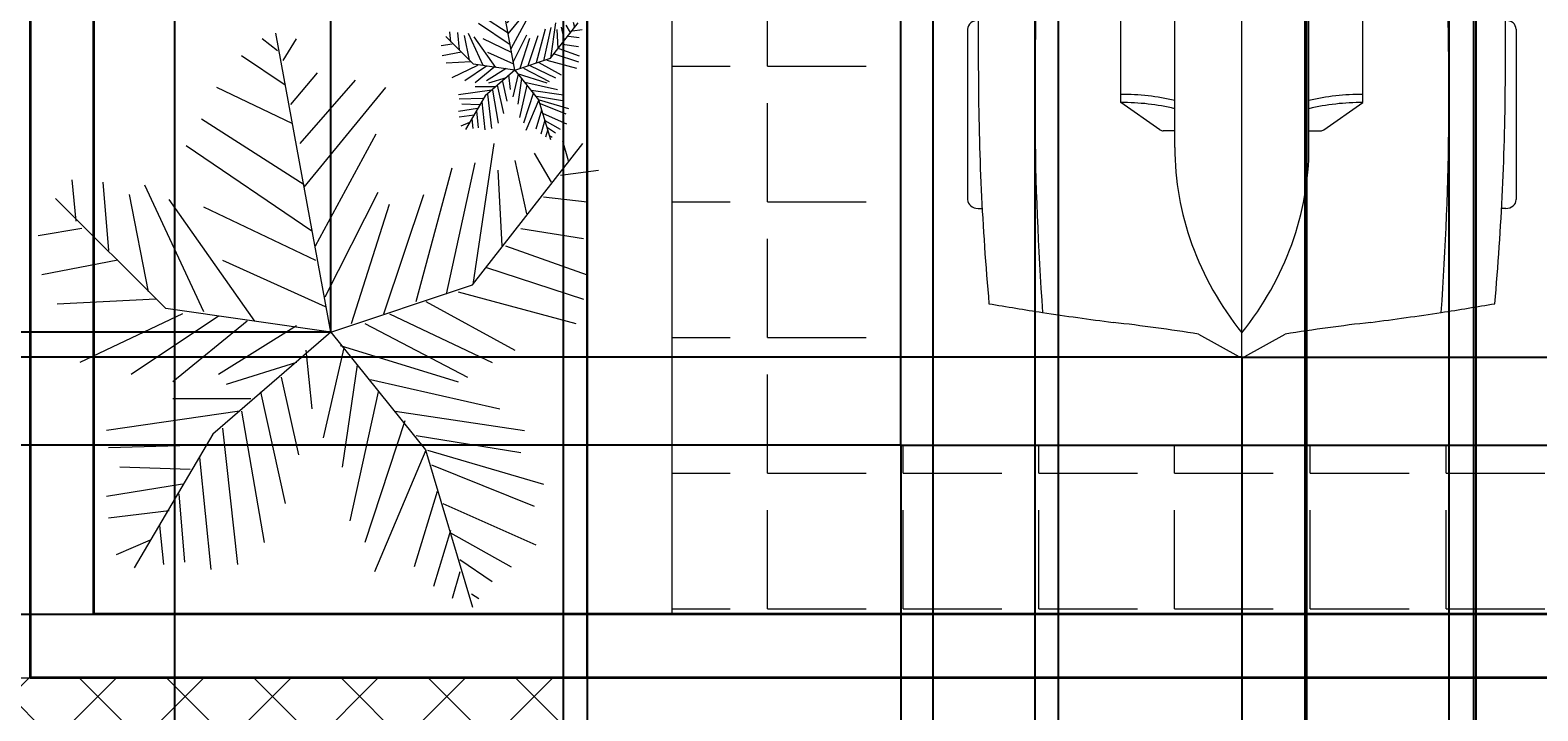
# Model space of a CAD drawing. Units: inches. Extents: x 818 to 1898, y 976 to 2364.
# Tile 3 of 96: x 993 to 1207, y 1198 to 1295. Entities that reach past the tile are written whole.
import ezdxf

# ---------------------------------------------------------------- set-up
doc = ezdxf.new("R2010")
doc.units = ezdxf.units.IN
doc.header["$LTSCALE"] = 5
doc.header["$MEASUREMENT"] = 0
for name, color, linetype, lineweight in [('A-ANNO-DIMS', 2, 'Continuous', 18), ('C-PAVE-PATT', 8, 'Continuous', 9), ('C-PKNG', 8, 'Continuous', 18), ('C-PKNG-PATT', 9, 'Continuous', 9), ('C-PROP', 7, 'Continuous', 35), ('L-PAVE', 8, 'Continuous', 18), ('L-PLNT-BEDS', 94, 'Continuous', 18)]:
    doc.layers.add(name, color=color, linetype=linetype, lineweight=lineweight)
doc.layers.add('L-PLNT', color=116, linetype='Continuous', lineweight=13, true_color=0x136734)
doc.styles.get("Standard").update_dxf_attribs({"font": 'arial.ttf'})
doc.dimstyles.get("Standard").update_dxf_attribs({"dimtxt": 0.18, "dimasz": 0.18, "dimexe": 0.18, "dimexo": 0.0625, "dimgap": 0.09, "dimtad": 0, "dimtih": 1, "dimtoh": 1, "dimdec": 4, "dimzin": 0, "dimdsep": 46, "dimtxsty": 'Standard', "dimcen": 0.09, "dimadec": 0, "dimazin": 0, "dimtfac": 1, "dimtdec": 4, "dimtofl": 0, "dimtmove": 0, "dimatfit": 3, "dimfxl": 1, "dimtolj": 1, "dimtzin": 0, "dimarcsym": 0})
pattern_1 = [(0, (0, 0), (0, 19.25), [14, -5.25]), (90, (0, 0), (-19.25, 1e-15), [14, -5.25])]

# ---------------------------------------------------------------- blocks, each defined once
blk = doc.blocks.new('*U13')
for p, q in [((46.55, 38.89), (22.35, 38.89)), ((136.7, 38.89), (160.9, 38.89)), ((21.1, 37.41), (21.1, 36.83)), ((47.8, 37.39), (47.8, 37.41)), ((135.45, 37.07), (135.45, 37.41)), ((162.15, 37.41), (162.15, 36.77)), ((87.99, 31.87), (74.76, 35.92)), ((134.31, 35.6), (119.29, 31.78)), ((186.47, -33.5), (186.47, 33.5)), ((188.4, -32.76), (188.4, 32.76)), ((70.03, 31.54), (86.41, 29.35)), ((138.42, 29.35), (157.25, 29.35)), ((186.47, 29.35), (167.01, 29.35)), ((164.52, 26.39), (164.52, -26.39)), ((32.27, 11.63), (36.13, 17.17)), ((36.13, 17.17), (50.94, 17.17)), ((32.12, 9.51), (32.12, 11.15)), ((58.92, -10.77), (58.92, 10.77)), ((29.77, 9.51), (51.68, 9.51)), ((66.55, -10.53), (66.55, 10.53)), ((186.47, -10.53), (186.47, 10.53)), ((82.74, 8.5), (82.74, -8.5)), ((3.27, 6.13), (0.1, 0.41)), ((0, 0), (51.68, 0)), ((0.1, -0.41), (3.27, -6.13)), ((29.77, -9.51), (51.68, -9.51)), ((32.12, -9.51), (32.12, -11.15)), ((32.27, -11.63), (36.13, -17.17)), ((36.13, -17.17), (50.94, -17.17)), ((86.41, -29.35), (70.03, -31.54)), ((157.25, -29.35), (138.42, -29.35)), ((167.01, -29.35), (186.47, -29.35)), ((87.99, -31.87), (74.76, -35.92)), ((134.31, -35.6), (119.29, -31.78)), ((21.1, -37.41), (21.1, -36.83)), ((47.8, -37.39), (47.8, -37.41)), ((135.45, -37.07), (135.45, -37.41)), ((162.15, -37.41), (162.15, -36.77)), ((46.55, -38.89), (22.35, -38.89)), ((136.7, -38.89), (160.9, -38.89))]:
    blk.add_line(p, q)
for centre, major_axis, ratio, start_param, end_param in [((22.35, 37.41), (0, -1.48), 0.842304, 3.141593, 4.712389), ((46.55, 37.41), (0, 1.48), 0.842304, -1.570796, 0), ((136.7, 37.41), (0, -1.48), 0.842304, 3.141593, 4.712389), ((160.9, 37.41), (0, 1.48), 0.842304, -1.570796, 0), ((41.19, -490.86), (0, 528.23), 0.842304, 0.00281, 0.075598), ((64.48, -10555.62), (0, 10593.03), 0.842304, -0.013397, 0.002797), ((180.63, 35.84), (0, 2.22), 0.842304, -0.013017, 1.249894), ((64.48, -10556.36), (0, 10595.31), 0.842304, -0.013397, -0.013017), ((183.98, 33.5), (0, -2.96), 0.842304, 1.570796, 3.128196), ((183.98, 32.76), (0, -5.25), 0.842304, 1.570796, 3.128196), ((266.03, -27.52), (0, 313.31), 0.842304, 1.367076, 1.39176), ((64.48, -10555.62), (0, -10591.55), 0.842304, 3.133765, 3.140441), ((135.29, 5.39), (0, 81.77), 0.842304, 1.245306, 1.50788), ((95.79, -3666.35), (0, -3698.24), 0.842304, 3.134049, 3.144098), ((259.18, -27.52), (0, -305.3), 0.842304, 4.528606, 4.561838), ((37.47, -593.96), (0, -623.33), 0.842304, 3.096046, 3.200911), ((134.4, 5.39), (0, -89.78), 0.842304, 4.449482, 4.652344), ((149.6, 2.8), (0, -79.58), 0.842304, 4.372215, 4.640744), ((17.08, 0), (0, 147.02), 0.842304, 4.511394, 4.913384), ((35.91, 0), (0, 147.02), 0.842304, 4.511394, 4.913384), ((167.01, 26.39), (0, 2.96), 0.842304, 0, 1.570796), ((-204.49, 52.4), (0, -250.96), 0.842304, 1.385369, 1.434372), ((13.04, 17.01), (0, 27.42), 0.842304, 4.435146, 4.718221), ((14.2, 17.01), (0, 27.42), 0.842304, 4.435146, 4.718221), ((50.79, 13.34), (6.34, -0.36), 0.603834, -1.395552, 1.581315), ((32.75, 11.15), (0, 0.74), 0.842304, 0.879714, 1.570796), ((29.77, -46.66), (0, 56.17), 0.842304, 0, 0.590319), ((0.62, 0), (0, -0.74), 0.842304, 4.131459, 5.293319), ((29.77, 46.66), (0, 56.17), 0.842304, 2.551274, 3.141593), ((-204.49, -52.4), (0, 250.96), 0.842304, -1.434372, -1.385369), ((149.6, -2.8), (0, -79.58), 0.842304, -1.499151, -1.230623), ((13.04, -17.01), (0, -27.42), 0.842304, 1.564964, 1.848039), ((14.2, -17.01), (0, -27.42), 0.842304, 1.564964, 1.848039), ((135.29, -5.39), (0, -81.77), 0.842304, -1.50788, -1.245306), ((32.75, -11.15), (0, -0.74), 0.842304, 4.712389, 5.403472), ((134.4, -5.39), (0, -89.78), 0.842304, -1.510751, -1.307889), ((259.18, 27.52), (0, 305.3), 0.842304, 1.721348, 1.754579), ((167.01, -26.39), (0, -2.96), 0.842304, 4.712389, 6.283185), ((266.03, 27.52), (0, 313.31), 0.842304, 1.749832, 1.774517), ((37.47, 593.96), (0, -623.33), 0.842304, -0.059319, 0.045547), ((95.79, 3666.35), (0, -3698.24), 0.842304, -0.002505, 0.007544), ((183.98, -33.5), (0, 2.96), 0.842304, 3.15499, 4.712389), ((183.98, -32.76), (0, -5.25), 0.842304, 0.013397, 1.570796), ((41.19, 490.86), (0, -528.23), 0.842304, -0.075598, -0.00281), ((64.48, 10555.62), (0, -10591.55), 0.842304, 0.001152, 0.007828), ((22.35, -37.41), (0, 1.48), 0.842304, 1.570796, 3.141593), ((64.48, 10555.62), (0, 10593.03), 0.842304, 3.138796, 3.15499), ((46.55, -37.41), (0, -1.48), 0.842304, 0, 1.570796), ((136.7, -37.41), (0, -1.48), 0.842304, -1.570796, 0), ((160.9, -37.41), (0, 1.48), 0.842304, 3.141593, 4.712389), ((180.63, -35.84), (0, -2.22), 0.842304, -1.249894, 0.013017), ((64.48, 10556.36), (0, 10595.31), 0.842304, 3.15461, 3.15499)]:
    blk.add_ellipse(centre, major_axis=major_axis, ratio=ratio, start_param=start_param, end_param=end_param)
at = {"extrusion": (0, 0, -1)}
blk.add_ellipse((50.79, -13.34), major_axis=(6.34, 0.36), ratio=0.603834, start_param=-1.395552, end_param=1.581315, dxfattribs=at)
blk = doc.blocks.new('SHRUB-ACCENT')
for p, q in [((8.8, 18.63), (7.25, 19.67)), ((8.53, 19.84), (7.99, 20.28)), ((10.44, 9.82), (8.47, 20.47)), ((8.74, 19.5), (9.21, 20.28)), ((9.48, 15.07), (5.82, 17.41)), ((9.08, 17.24), (6.37, 18.54)), ((9.01, 17.93), (9.96, 19.06)), ((9.35, 16.54), (11.31, 18.8)), ((9.48, 14.98), (12.39, 18.54)), ((1.35, 13.77), (1.22, 15.24)), ((2.3, 15.16), (2.51, 12.72)), ((3.79, 15.07), (5.89, 10.55)), ((9.75, 13.42), (5.28, 16.46)), ((9.89, 12.9), (12.06, 16.89)), ((13.48, 10.9), (14.76, 15.68)), ((14.56, 11.16), (15.58, 15.85)), ((15.49, 11.5), (19.41, 16.55)), ((15.51, 11.51), (16.25, 16.54)), ((16.39, 15.59), (16.53, 12.9)), ((17, 15.94), (17.41, 14.03)), ((17.68, 16.2), (18.29, 15.16)), ((18.62, 15.42), (19.98, 15.59)), ((18.69, 16.63), (18.9, 15.94)), ((1.56, 13.51), (0, 13.25)), ((4.55, 10.66), (0.62, 14.58)), ((3.25, 14.72), (3.93, 11.25)), ((7.72, 10.21), (4.67, 14.55)), ((5.89, 14.29), (9.89, 12.38)), ((10.23, 11.07), (12.12, 14.81)), ((11.17, 10.12), (12.53, 14.37)), ((12.33, 10.47), (13.75, 14.72)), ((16.66, 12.9), (19.57, 11.86)), ((17.2, 13.51), (19.44, 13.16)), ((18.02, 14.63), (19.57, 14.46)), ((2.84, 12.38), (0.14, 11.86)), ((4.2, 10.99), (0.68, 10.81)), ((6.57, 12.38), (10.23, 10.73)), ((10.44, 9.82), (15.49, 11.5)), ((13.82, 10.9), (17, 9.16)), ((14.97, 11.25), (19.17, 10.12)), ((15.98, 12.12), (19.44, 10.99)), ((5.15, 10.47), (1.49, 8.73)), ((6.43, 10.38), (3.32, 8.3)), ((10.44, 9.82), (4.55, 10.66)), ((7.45, 10.21), (4.81, 8.04)), ((10.44, 9.82), (6.23, 6.17)), ((9.21, 10.03), (6.43, 8.3)), ((9.21, 8.73), (6.7, 7.95)), ((9.55, 9.16), (9.75, 7.08)), ((10.9, 9.25), (10.16, 6.04)), ((10.44, 9.82), (13.8, 5.61)), ((10.77, 9.34), (14.97, 8.04)), ((11.38, 8.64), (10.84, 5)), ((11.65, 10.12), (15.31, 8.21)), ((12.53, 10.47), (16.19, 8.73)), ((7.18, 6.99), (2.44, 6.3)), ((7.59, 7.43), (4.81, 7.43)), ((7.25, 6.99), (8.06, 2.31)), ((7.92, 7.69), (8.8, 3.69)), ((8.67, 8.21), (9.28, 5.43)), ((12.12, 7.69), (11.11, 3.09)), ((13.07, 6.65), (11.65, 2.31)), ((11.85, 8.12), (16.46, 7.08)), ((12.73, 6.99), (17.34, 6.3)), ((5.15, 4.39), (2.44, 3.95)), ((5.89, 5.78), (2.51, 5.69)), ((5.42, 4.91), (2.91, 5)), ((6.23, 6.17), (3.43, 1.4)), ((5.76, 5.34), (6.16, 1.35)), ((6.57, 6.39), (7.11, 1.52)), ((13.82, 5.6), (11.99, 1.26)), ((13.48, 6.13), (17.2, 5.52)), ((13.8, 5.61), (15.49, 0)), ((13.88, 5.6), (18.02, 4.39)), ((14.02, 5.08), (17.68, 3.61)), ((4.67, 3.43), (2.51, 3.17)), ((4, 2.39), (2.78, 1.87)), ((4.33, 2.91), (4.47, 1.52)), ((5.01, 4.04), (5.21, 1.61)), ((14.22, 4.13), (13.41, 1.44)), ((14.7, 2.74), (14.09, 0.74)), ((14.43, 3.69), (17.74, 2.22)), ((14.7, 2.65), (16.86, 1.44)), ((15.04, 1.26), (14.76, 0.31)), ((15.04, 1.7), (16.19, 0.92)), ((15.44, 0.48), (15.71, 0.31))]:
    blk.add_line(p, q)
blk = doc.blocks.new('PALM-BORDER')
for p, q in [((41.53, 39.05), (33.72, 81.45)), ((33.95, 78.95), (31.8, 80.68)), ((34.76, 77.57), (36.65, 80.68)), ((35.03, 74.11), (28.83, 78.26)), ((35.84, 71.35), (39.61, 75.84)), ((36.11, 68.59), (25.33, 73.77)), ((37.18, 65.82), (45, 74.8)), ((37.72, 59.6), (49.31, 73.77)), ((37.72, 59.95), (23.17, 69.28)), ((39.34, 51.31), (47.96, 67.2)), ((38.8, 53.39), (21.02, 65.48)), ((61.61, 45.75), (77.23, 65.83)), ((61.71, 45.79), (64.67, 65.82)), ((70.33, 64.44), (72.75, 60.3)), ((74.37, 66.17), (75.18, 63.4)), ((53.62, 43.37), (58.74, 62.37)), ((57.93, 44.41), (61.97, 63.06)), ((65.21, 62.02), (65.75, 51.31)), ((67.63, 63.4), (69.25, 55.81)), ((74.1, 61.33), (79.49, 62.02)), ((5.39, 54.77), (4.85, 60.64)), ((9.16, 60.3), (9.97, 50.62)), ((15.09, 59.95), (23.44, 41.99)), ((18.1, 42.4), (2.48, 58.02)), ((12.93, 58.57), (15.63, 44.75)), ((30.72, 40.61), (18.59, 57.88)), ((40.69, 44.06), (48.23, 58.91)), ((49.04, 41.64), (54.7, 58.57)), ((71.68, 58.22), (77.87, 57.53)), ((23.44, 56.84), (39.34, 49.24)), ((44.46, 40.26), (49.85, 57.19)), ((6.2, 53.73), (0, 52.7)), ((68.44, 53.73), (77.33, 52.35)), ((66.29, 51.31), (77.87, 47.17)), ((11.32, 49.24), (0.54, 47.17)), ((26.14, 49.24), (40.69, 42.68)), ((63.59, 48.21), (77.33, 43.71)), ((41.53, 39.05), (61.61, 45.75)), ((16.71, 43.71), (2.69, 43.02)), ((54.97, 43.37), (67.63, 36.46)), ((59.55, 44.75), (76.26, 40.26)), ((20.48, 41.64), (5.93, 34.73)), ((25.6, 41.3), (13.2, 33.01)), ((41.53, 39.05), (18.1, 42.4)), ((49.85, 41.64), (64.4, 34.73)), ((29.64, 40.61), (19.13, 31.97)), ((41.53, 39.05), (24.79, 24.55)), ((36.65, 39.91), (25.6, 33.01)), ((41.53, 39.05), (54.92, 22.32)), ((46.35, 40.26), (60.9, 32.66)), ((37.99, 36.46), (38.8, 28.17)), ((43.38, 36.81), (40.42, 24.02)), ((42.84, 37.15), (59.55, 31.97)), ((36.65, 34.73), (26.68, 31.62)), ((45.27, 34.39), (43.11, 19.88)), ((34.49, 32.66), (36.92, 21.61)), ((47.15, 32.32), (65.48, 28.17)), ((31.53, 30.59), (35.03, 14.7)), ((48.23, 30.59), (44.19, 12.28)), ((28.56, 27.82), (9.7, 25.06)), ((30.18, 29.55), (19.13, 29.55)), ((28.83, 27.82), (32.07, 9.17)), ((50.66, 27.82), (68.98, 25.06)), ((52, 26.44), (46.35, 9.17)), ((24.79, 24.55), (13.63, 5.58)), ((26.14, 25.41), (28.29, 6.06)), ((53.62, 24.37), (68.44, 21.95)), ((23.44, 22.99), (9.97, 22.64)), ((54.97, 22.3), (47.69, 5.02)), ((54.92, 22.32), (61.61, 0)), ((55.24, 22.3), (71.68, 17.46)), ((21.56, 19.53), (11.59, 19.88)), ((22.9, 21.26), (24.52, 5.37)), ((55.78, 20.22), (70.33, 14.35)), ((20.48, 17.46), (9.7, 15.73)), ((19.94, 16.08), (20.75, 6.41)), ((56.59, 16.42), (53.35, 5.72)), ((18.59, 13.66), (9.97, 12.62)), ((57.39, 14.7), (70.6, 8.83)), ((17.24, 11.59), (17.78, 6.06)), ((58.47, 10.9), (56.05, 2.95)), ((15.9, 9.52), (11.05, 7.44)), ((58.47, 10.55), (67.09, 5.72)), ((59.82, 6.75), (64.4, 3.64)), ((59.82, 5.02), (58.74, 1.22)), ((61.44, 1.92), (62.51, 1.22))]:
    blk.add_line(p, q)
blk = doc.blocks.new('*D59')
at = {"layer": 'A-ANNO-DIMS', "color": 0, "lineweight": -2, "ltscale": 5, "transparency": 16777216}
for p, q in [((1251.64, 2300.39), (818.03, 2300.39)), ((818.21, 2300.21), (818.21, 1669.95)), ((818.21, 1039.32), (818.21, 1669.59)), ((896.05, 1039.14), (818.03, 1039.14))]:
    blk.add_line(p, q, dxfattribs=at)
at = {"layer": 'A-ANNO-DIMS', "color": 0, "ltscale": 5, "transparency": 16777216}
for points in [[(818.18, 2300.21), (818.24, 2300.21), (818.21, 2300.39)], [(818.18, 1039.32), (818.24, 1039.32), (818.21, 1039.14)]]:
    blk.add_solid(points, dxfattribs=at)
at = {"layer": 'Defpoints', "color": 0, "ltscale": 5, "transparency": 16777216}
for p in [(818.21, 2300.39), (1251.71, 2300.39), (896.11, 1039.14)]:
    blk.add_point(p, dxfattribs=at)
at = {"layer": 'A-ANNO-DIMS', "color": 0, "ltscale": 5, "transparency": 16777216, "insert": (818.21, 1669.77), "char_height": 0.18, "attachment_point": 5}
blk.add_mtext('\\A1;1261.2', dxfattribs=at)
blk = doc.blocks.new('*D61')
at = {"layer": 'A-ANNO-DIMS', "color": 0, "lineweight": -2, "ltscale": 5, "transparency": 16777216}
for p, q in [((1071.73, 1203.03), (1071.73, 2363.87)), ((1071.91, 2363.69), (1250.94, 2363.69)), ((1430.55, 2363.69), (1251.51, 2363.69)), ((1430.73, 1203.03), (1430.73, 2363.87))]:
    blk.add_line(p, q, dxfattribs=at)
at = {"layer": 'A-ANNO-DIMS', "color": 0, "ltscale": 5, "transparency": 16777216}
for points in [[(1071.91, 2363.72), (1071.91, 2363.66), (1071.73, 2363.69)], [(1430.55, 2363.72), (1430.55, 2363.66), (1430.73, 2363.69)]]:
    blk.add_solid(points, dxfattribs=at)
at = {"layer": 'Defpoints', "color": 0, "ltscale": 5, "transparency": 16777216}
for p in [(1430.73, 2363.69), (1071.73, 1202.96), (1430.73, 1202.96)]:
    blk.add_point(p, dxfattribs=at)
at = {"layer": 'A-ANNO-DIMS', "color": 0, "ltscale": 5, "transparency": 16777216, "insert": (1251.23, 2363.69), "char_height": 0.18, "attachment_point": 5}
blk.add_mtext('\\A1;359', dxfattribs=at)
blk = doc.blocks.new('*D62')
at = {"layer": 'A-ANNO-DIMS', "color": 0, "lineweight": -2, "ltscale": 5, "transparency": 16777216}
for p, q in [((1116.19, 1235.9), (1116.19, 975.66)), ((1406.73, 1235.9), (1406.73, 975.66)), ((1116.37, 975.84), (1260.99, 975.84)), ((1406.55, 975.84), (1261.92, 975.84))]:
    blk.add_line(p, q, dxfattribs=at)
at = {"layer": 'A-ANNO-DIMS', "color": 0, "ltscale": 5, "transparency": 16777216}
for points in [[(1116.37, 975.87), (1116.37, 975.81), (1116.19, 975.84)], [(1406.55, 975.87), (1406.55, 975.81), (1406.73, 975.84)]]:
    blk.add_solid(points, dxfattribs=at)
at = {"layer": 'Defpoints', "color": 0, "ltscale": 5, "transparency": 16777216}
for p in [(1116.19, 1235.96), (1406.73, 1235.96), (1406.73, 975.84)]:
    blk.add_point(p, dxfattribs=at)
at = {"layer": 'A-ANNO-DIMS', "color": 0, "ltscale": 5, "transparency": 16777216, "insert": (1261.46, 975.84), "char_height": 0.18, "attachment_point": 5}
blk.add_mtext('\\A1;290.54', dxfattribs=at)
blk = doc.blocks.new('*D63')
at = {"layer": 'A-ANNO-DIMS', "color": 0, "lineweight": -2, "ltscale": 5, "transparency": 16777216}
for p, q in [((1116.13, 1485.2), (818.03, 1485.2)), ((818.21, 1485.02), (818.21, 1360.77)), ((818.21, 1236.14), (818.21, 1360.4)), ((1116.13, 1235.96), (818.03, 1235.96))]:
    blk.add_line(p, q, dxfattribs=at)
at = {"layer": 'A-ANNO-DIMS', "color": 0, "ltscale": 5, "transparency": 16777216}
for points in [[(818.18, 1485.02), (818.24, 1485.02), (818.21, 1485.2)], [(818.18, 1236.14), (818.24, 1236.14), (818.21, 1235.96)]]:
    blk.add_solid(points, dxfattribs=at)
at = {"layer": 'Defpoints', "color": 0, "ltscale": 5, "transparency": 16777216}
for p in [(818.21, 1485.2), (1116.19, 1485.2), (1116.19, 1235.96)]:
    blk.add_point(p, dxfattribs=at)
at = {"layer": 'A-ANNO-DIMS', "color": 0, "ltscale": 5, "transparency": 16777216, "insert": (818.21, 1360.58), "char_height": 0.18, "attachment_point": 5}
blk.add_mtext('\\A1;249.24', dxfattribs=at)
blk = doc.blocks.new('*D79')
at = {"layer": 'A-ANNO-DIMS', "color": 0, "lineweight": -2, "ltscale": 5, "transparency": 16777216}
for p, q in [((992.73, 1203.03), (992.73, 2363.87)), ((992.91, 2363.69), (1032.01, 2363.69)), ((1071.55, 2363.69), (1032.44, 2363.69)), ((1071.73, 1203.03), (1071.73, 2363.87))]:
    blk.add_line(p, q, dxfattribs=at)
at = {"layer": 'A-ANNO-DIMS', "color": 0, "ltscale": 5, "transparency": 16777216}
for points in [[(992.91, 2363.72), (992.91, 2363.66), (992.73, 2363.69)], [(1071.55, 2363.72), (1071.55, 2363.66), (1071.73, 2363.69)]]:
    blk.add_solid(points, dxfattribs=at)
at = {"layer": 'Defpoints', "color": 0, "ltscale": 5, "transparency": 16777216}
for p in [(1071.73, 2363.69), (992.73, 1202.96), (1071.73, 1202.96)]:
    blk.add_point(p, dxfattribs=at)
at = {"layer": 'A-ANNO-DIMS', "color": 0, "ltscale": 5, "transparency": 16777216, "insert": (1032.23, 2363.69), "char_height": 0.18, "attachment_point": 5}
blk.add_mtext('\\A1;79', dxfattribs=at)
blk = doc.blocks.new('*D80')
at = {"layer": 'A-ANNO-DIMS', "color": 0, "lineweight": -2, "ltscale": 5, "transparency": 16777216}
for p, q in [((1116.19, 1235.9), (1116.19, 975.66)), ((1071.73, 1202.9), (1071.73, 975.66)), ((1071.91, 975.84), (1093.56, 975.84)), ((1116.01, 975.84), (1094.35, 975.84))]:
    blk.add_line(p, q, dxfattribs=at)
at = {"layer": 'A-ANNO-DIMS', "color": 0, "ltscale": 5, "transparency": 16777216}
for points in [[(1071.91, 975.87), (1071.91, 975.81), (1071.73, 975.84)], [(1116.01, 975.87), (1116.01, 975.81), (1116.19, 975.84)]]:
    blk.add_solid(points, dxfattribs=at)
at = {"layer": 'Defpoints', "color": 0, "ltscale": 5, "transparency": 16777216}
for p in [(1116.19, 1235.96), (1071.73, 1202.96), (1116.19, 975.84)]:
    blk.add_point(p, dxfattribs=at)
at = {"layer": 'A-ANNO-DIMS', "color": 0, "ltscale": 5, "transparency": 16777216, "insert": (1093.96, 975.84), "char_height": 0.18, "attachment_point": 5}
blk.add_mtext('\\A1;44.46', dxfattribs=at)
blk = doc.blocks.new('*D81')
at = {"layer": 'A-ANNO-DIMS', "color": 0, "lineweight": -2, "ltscale": 5, "transparency": 16777216}
for p, q in [((1116.13, 1235.96), (818.03, 1235.96)), ((818.21, 1235.78), (818.21, 1224.14)), ((818.21, 1212.14), (818.21, 1223.78)), ((1083.66, 1211.96), (818.03, 1211.96))]:
    blk.add_line(p, q, dxfattribs=at)
at = {"layer": 'A-ANNO-DIMS', "color": 0, "ltscale": 5, "transparency": 16777216}
for points in [[(818.18, 1235.78), (818.24, 1235.78), (818.21, 1235.96)], [(818.18, 1212.14), (818.24, 1212.14), (818.21, 1211.96)]]:
    blk.add_solid(points, dxfattribs=at)
at = {"layer": 'Defpoints', "color": 0, "ltscale": 5, "transparency": 16777216}
for p in [(1116.19, 1235.96), (818.21, 1211.96), (1083.73, 1211.96)]:
    blk.add_point(p, dxfattribs=at)
at = {"layer": 'A-ANNO-DIMS', "color": 0, "ltscale": 5, "transparency": 16777216, "insert": (818.21, 1223.96), "char_height": 0.18, "attachment_point": 5}
blk.add_mtext('\\A1;24', dxfattribs=at)
blk = doc.blocks.new('*D91')
at = {"layer": 'A-ANNO-DIMS', "color": 0, "lineweight": -2, "ltscale": 5, "transparency": 16777216}
for p, q in [((959.17, 1071.12), (959.17, 2363.87)), ((959.35, 2363.69), (985.8, 2363.69)), ((1013.04, 2363.69), (986.59, 2363.69)), ((1013.22, 1071.12), (1013.22, 2363.87))]:
    blk.add_line(p, q, dxfattribs=at)
at = {"layer": 'A-ANNO-DIMS', "color": 0, "ltscale": 5, "transparency": 16777216}
for points in [[(959.35, 2363.72), (959.35, 2363.66), (959.17, 2363.69)], [(1013.04, 2363.72), (1013.04, 2363.66), (1013.22, 2363.69)]]:
    blk.add_solid(points, dxfattribs=at)
at = {"layer": 'Defpoints', "color": 0, "ltscale": 5, "transparency": 16777216}
for p in [(1013.22, 2363.69), (959.17, 1071.06), (1013.22, 1071.06)]:
    blk.add_point(p, dxfattribs=at)
at = {"layer": 'A-ANNO-DIMS', "color": 0, "ltscale": 5, "transparency": 16777216, "insert": (986.2, 2363.69), "char_height": 0.18, "attachment_point": 5}
blk.add_mtext('\\A1;54.04', dxfattribs=at)
blk = doc.blocks.new('*D92')
at = {"layer": 'A-ANNO-DIMS', "color": 0, "lineweight": -2, "ltscale": 5, "transparency": 16777216}
for p, q in [((1013.22, 1071.12), (1013.22, 2363.87)), ((1013.4, 2363.69), (1040.38, 2363.69)), ((1068.16, 2363.69), (1041.17, 2363.69)), ((1068.34, 1071.12), (1068.34, 2363.87))]:
    blk.add_line(p, q, dxfattribs=at)
at = {"layer": 'A-ANNO-DIMS', "color": 0, "ltscale": 5, "transparency": 16777216}
for points in [[(1013.4, 2363.72), (1013.4, 2363.66), (1013.22, 2363.69)], [(1068.16, 2363.72), (1068.16, 2363.66), (1068.34, 2363.69)]]:
    blk.add_solid(points, dxfattribs=at)
at = {"layer": 'Defpoints', "color": 0, "ltscale": 5, "transparency": 16777216}
for p in [(1068.34, 2363.69), (1013.22, 1071.06), (1068.34, 1071.06)]:
    blk.add_point(p, dxfattribs=at)
at = {"layer": 'A-ANNO-DIMS', "color": 0, "ltscale": 5, "transparency": 16777216, "insert": (1040.78, 2363.69), "char_height": 0.18, "attachment_point": 5}
blk.add_mtext('\\A1;55.12', dxfattribs=at)
blk = doc.blocks.new('*D93')
at = {"layer": 'A-ANNO-DIMS', "color": 0, "lineweight": -2, "ltscale": 5, "transparency": 16777216}
for p, q in [((1068.34, 1071.12), (1068.34, 2363.87)), ((1068.52, 2363.69), (1094.16, 2363.69)), ((1120.58, 2363.69), (1094.94, 2363.69)), ((1120.76, 1071.12), (1120.76, 2363.87))]:
    blk.add_line(p, q, dxfattribs=at)
at = {"layer": 'A-ANNO-DIMS', "color": 0, "ltscale": 5, "transparency": 16777216}
for points in [[(1068.52, 2363.72), (1068.52, 2363.66), (1068.34, 2363.69)], [(1120.58, 2363.72), (1120.58, 2363.66), (1120.76, 2363.69)]]:
    blk.add_solid(points, dxfattribs=at)
at = {"layer": 'Defpoints', "color": 0, "ltscale": 5, "transparency": 16777216}
for p in [(1120.76, 2363.69), (1068.34, 1071.06), (1120.76, 1071.06)]:
    blk.add_point(p, dxfattribs=at)
at = {"layer": 'A-ANNO-DIMS', "color": 0, "ltscale": 5, "transparency": 16777216, "insert": (1094.55, 2363.69), "char_height": 0.18, "attachment_point": 5}
blk.add_mtext('\\A1;52.42', dxfattribs=at)
blk = doc.blocks.new('*D94')
at = {"layer": 'A-ANNO-DIMS', "color": 0, "lineweight": -2, "ltscale": 5, "transparency": 16777216}
for p, q in [((1120.76, 1071.12), (1120.76, 2363.87)), ((1120.94, 2363.69), (1146.76, 2363.69)), ((1173.36, 2363.69), (1147.55, 2363.69)), ((1173.54, 1071.12), (1173.54, 2363.87))]:
    blk.add_line(p, q, dxfattribs=at)
at = {"layer": 'A-ANNO-DIMS', "color": 0, "ltscale": 5, "transparency": 16777216}
for points in [[(1120.94, 2363.72), (1120.94, 2363.66), (1120.76, 2363.69)], [(1173.36, 2363.72), (1173.36, 2363.66), (1173.54, 2363.69)]]:
    blk.add_solid(points, dxfattribs=at)
at = {"layer": 'Defpoints', "color": 0, "ltscale": 5, "transparency": 16777216}
for p in [(1173.54, 2363.69), (1120.76, 1071.06), (1173.54, 1071.06)]:
    blk.add_point(p, dxfattribs=at)
at = {"layer": 'A-ANNO-DIMS', "color": 0, "ltscale": 5, "transparency": 16777216, "insert": (1147.15, 2363.69), "char_height": 0.18, "attachment_point": 5}
blk.add_mtext('\\A1;52.78', dxfattribs=at)
blk = doc.blocks.new('*D95')
at = {"layer": 'A-ANNO-DIMS', "color": 0, "lineweight": -2, "ltscale": 5, "transparency": 16777216}
for p, q in [((1173.54, 1071.12), (1173.54, 2363.87)), ((1173.72, 2363.69), (1201.29, 2363.69)), ((1229.47, 2363.69), (1201.9, 2363.69)), ((1229.65, 1071.12), (1229.65, 2363.87))]:
    blk.add_line(p, q, dxfattribs=at)
at = {"layer": 'A-ANNO-DIMS', "color": 0, "ltscale": 5, "transparency": 16777216}
for points in [[(1173.72, 2363.72), (1173.72, 2363.66), (1173.54, 2363.69)], [(1229.47, 2363.72), (1229.47, 2363.66), (1229.65, 2363.69)]]:
    blk.add_solid(points, dxfattribs=at)
at = {"layer": 'Defpoints', "color": 0, "ltscale": 5, "transparency": 16777216}
for p in [(1229.65, 2363.69), (1173.54, 1071.06), (1229.65, 1071.06)]:
    blk.add_point(p, dxfattribs=at)
at = {"layer": 'A-ANNO-DIMS', "color": 0, "ltscale": 5, "transparency": 16777216, "insert": (1201.59, 2363.69), "char_height": 0.18, "attachment_point": 5}
blk.add_mtext('\\A1;56.1', dxfattribs=at)
blk = doc.blocks.new('*D105')
at = {"layer": 'A-ANNO-DIMS', "color": 0, "lineweight": -2, "ltscale": 5, "transparency": 16777216}
for p, q in [((1164.56, 1248.4), (1164.56, 975.66)), ((1116.19, 1235.9), (1116.19, 975.66)), ((1116.37, 975.84), (1139.98, 975.84)), ((1164.38, 975.84), (1140.77, 975.84))]:
    blk.add_line(p, q, dxfattribs=at)
at = {"layer": 'A-ANNO-DIMS', "color": 0, "ltscale": 5, "transparency": 16777216}
for points in [[(1116.37, 975.87), (1116.37, 975.81), (1116.19, 975.84)], [(1164.38, 975.87), (1164.38, 975.81), (1164.56, 975.84)]]:
    blk.add_solid(points, dxfattribs=at)
at = {"layer": 'Defpoints', "color": 0, "ltscale": 5, "transparency": 16777216}
for p in [(1164.56, 1248.46), (1116.19, 1235.96), (1164.56, 975.84)]:
    blk.add_point(p, dxfattribs=at)
at = {"layer": 'A-ANNO-DIMS', "color": 0, "ltscale": 5, "transparency": 16777216, "insert": (1140.37, 975.84), "char_height": 0.18, "attachment_point": 5}
blk.add_mtext('\\A1;48.37', dxfattribs=at)
blk = doc.blocks.new('*D106')
at = {"layer": 'A-ANNO-DIMS', "color": 0, "lineweight": -2, "ltscale": 5, "transparency": 16777216}
for p, q in [((1164.56, 1248.4), (1164.56, 975.66)), ((1252.11, 1248.4), (1252.11, 975.66)), ((1164.74, 975.84), (1207.94, 975.84)), ((1251.93, 975.84), (1208.73, 975.84))]:
    blk.add_line(p, q, dxfattribs=at)
at = {"layer": 'A-ANNO-DIMS', "color": 0, "ltscale": 5, "transparency": 16777216}
for points in [[(1164.74, 975.87), (1164.74, 975.81), (1164.56, 975.84)], [(1251.93, 975.87), (1251.93, 975.81), (1252.11, 975.84)]]:
    blk.add_solid(points, dxfattribs=at)
at = {"layer": 'Defpoints', "color": 0, "ltscale": 5, "transparency": 16777216}
for p in [(1164.56, 1248.46), (1252.11, 1248.46), (1252.11, 975.84)]:
    blk.add_point(p, dxfattribs=at)
at = {"layer": 'A-ANNO-DIMS', "color": 0, "ltscale": 5, "transparency": 16777216, "insert": (1208.33, 975.84), "char_height": 0.18, "attachment_point": 5}
blk.add_mtext('\\A1;87.55', dxfattribs=at)
blk = doc.blocks.new('*D108')
at = {"layer": 'A-ANNO-DIMS', "color": 0, "lineweight": -2, "ltscale": 5, "transparency": 16777216}
for p, q in [((1131.74, 1436.86), (818.03, 1436.86)), ((818.21, 1436.68), (818.21, 1342.84)), ((818.21, 1248.64), (818.21, 1342.48)), ((1164.49, 1248.46), (818.03, 1248.46))]:
    blk.add_line(p, q, dxfattribs=at)
at = {"layer": 'A-ANNO-DIMS', "color": 0, "ltscale": 5, "transparency": 16777216}
for points in [[(818.18, 1436.68), (818.24, 1436.68), (818.21, 1436.86)], [(818.18, 1248.64), (818.24, 1248.64), (818.21, 1248.46)]]:
    blk.add_solid(points, dxfattribs=at)
at = {"layer": 'Defpoints', "color": 0, "ltscale": 5, "transparency": 16777216}
for p in [(818.21, 1436.86), (1131.8, 1436.86), (1164.56, 1248.46)]:
    blk.add_point(p, dxfattribs=at)
at = {"layer": 'A-ANNO-DIMS', "color": 0, "ltscale": 5, "transparency": 16777216, "insert": (818.21, 1342.66), "char_height": 0.18, "attachment_point": 5}
blk.add_mtext('\\A1;188.4', dxfattribs=at)
blk = doc.blocks.new('*D110')
at = {"layer": 'A-ANNO-DIMS', "color": 0, "lineweight": -2, "ltscale": 5, "transparency": 16777216}
for p, q in [((1164.62, 1248.46), (1897.92, 1248.46)), ((1897.74, 1248.28), (1897.74, 1242.4)), ((1897.74, 1236.14), (1897.74, 1242.03)), ((1116.25, 1235.96), (1897.92, 1235.96))]:
    blk.add_line(p, q, dxfattribs=at)
at = {"layer": 'A-ANNO-DIMS', "color": 0, "ltscale": 5, "transparency": 16777216}
for points in [[(1897.71, 1248.28), (1897.77, 1248.28), (1897.74, 1248.46)], [(1897.71, 1236.14), (1897.77, 1236.14), (1897.74, 1235.96)]]:
    blk.add_solid(points, dxfattribs=at)
at = {"layer": 'Defpoints', "color": 0, "ltscale": 5, "transparency": 16777216}
for p in [(1164.56, 1248.46), (1116.19, 1235.96), (1897.74, 1235.96)]:
    blk.add_point(p, dxfattribs=at)
at = {"layer": 'A-ANNO-DIMS', "color": 0, "ltscale": 5, "transparency": 16777216, "insert": (1897.74, 1242.21), "char_height": 0.18, "attachment_point": 5}
blk.add_mtext('\\A1;12.498', dxfattribs=at)
blk = doc.blocks.new('*D111')
at = {"layer": 'A-ANNO-DIMS', "color": 0, "lineweight": -2, "ltscale": 5, "transparency": 16777216}
for p, q in [((1135.21, 1405.65), (1135.21, 975.66)), ((1193.91, 1405.65), (1193.91, 975.66)), ((1135.39, 975.84), (1164.23, 975.84)), ((1193.73, 975.84), (1164.88, 975.84))]:
    blk.add_line(p, q, dxfattribs=at)
at = {"layer": 'A-ANNO-DIMS', "color": 0, "ltscale": 5, "transparency": 16777216}
for points in [[(1135.39, 975.87), (1135.39, 975.81), (1135.21, 975.84)], [(1193.73, 975.87), (1193.73, 975.81), (1193.91, 975.84)]]:
    blk.add_solid(points, dxfattribs=at)
at = {"layer": 'Defpoints', "color": 0, "ltscale": 5, "transparency": 16777216}
for p in [(1135.21, 1405.71), (1193.91, 1405.71), (1193.91, 975.84)]:
    blk.add_point(p, dxfattribs=at)
at = {"layer": 'A-ANNO-DIMS', "color": 0, "ltscale": 5, "transparency": 16777216, "insert": (1164.56, 975.84), "char_height": 0.18, "attachment_point": 5}
blk.add_mtext('\\A1;58.7', dxfattribs=at)
blk = doc.blocks.new('*D122')
at = {"layer": 'A-ANNO-DIMS', "color": 0, "lineweight": -2, "ltscale": 5, "transparency": 16777216}
for p, q in [((1138.5, 1794.37), (1138.5, 975.66)), ((1071.73, 1688.02), (1071.73, 975.66)), ((1071.91, 975.84), (1104.72, 975.84)), ((1138.32, 975.84), (1105.51, 975.84))]:
    blk.add_line(p, q, dxfattribs=at)
at = {"layer": 'A-ANNO-DIMS', "color": 0, "ltscale": 5, "transparency": 16777216}
for points in [[(1071.91, 975.87), (1071.91, 975.81), (1071.73, 975.84)], [(1138.32, 975.87), (1138.32, 975.81), (1138.5, 975.84)]]:
    blk.add_solid(points, dxfattribs=at)
at = {"layer": 'Defpoints', "color": 0, "ltscale": 5, "transparency": 16777216}
for p in [(1138.5, 1794.43), (1071.73, 1688.08), (1138.5, 975.84)]:
    blk.add_point(p, dxfattribs=at)
at = {"layer": 'A-ANNO-DIMS', "color": 0, "ltscale": 5, "transparency": 16777216, "insert": (1105.11, 975.84), "char_height": 0.18, "attachment_point": 5}
blk.add_mtext('\\A1;66.78', dxfattribs=at)
blk = doc.blocks.new('*D126')
at = {"layer": 'A-ANNO-DIMS', "color": 0, "lineweight": -2, "ltscale": 5, "transparency": 16777216}
for p, q in [((1035.38, 1252.09), (1035.38, 2363.87)), ((1035.56, 2363.69), (1075.41, 2363.69)), ((1116.01, 2363.69), (1076.16, 2363.69)), ((1116.19, 1236.03), (1116.19, 2363.87))]:
    blk.add_line(p, q, dxfattribs=at)
at = {"layer": 'A-ANNO-DIMS', "color": 0, "ltscale": 5, "transparency": 16777216}
for points in [[(1035.56, 2363.72), (1035.56, 2363.66), (1035.38, 2363.69)], [(1116.01, 2363.72), (1116.01, 2363.66), (1116.19, 2363.69)]]:
    blk.add_solid(points, dxfattribs=at)
at = {"layer": 'Defpoints', "color": 0, "ltscale": 5, "transparency": 16777216}
for p in [(1035.38, 2363.69), (1035.38, 1252.02), (1116.19, 1235.96)]:
    blk.add_point(p, dxfattribs=at)
at = {"layer": 'A-ANNO-DIMS', "color": 0, "ltscale": 5, "transparency": 16777216, "insert": (1075.78, 2363.69), "char_height": 0.18, "attachment_point": 5}
blk.add_mtext('\\A1;80.81', dxfattribs=at)
blk = doc.blocks.new('*D127')
at = {"layer": 'A-ANNO-DIMS', "color": 0, "lineweight": -2, "ltscale": 5, "transparency": 16777216}
for p, q in [((1035.31, 1252.02), (818.03, 1252.02)), ((818.21, 1251.84), (818.21, 1232.18)), ((818.21, 1212.14), (818.21, 1231.81)), ((1001.66, 1211.96), (818.03, 1211.96))]:
    blk.add_line(p, q, dxfattribs=at)
at = {"layer": 'A-ANNO-DIMS', "color": 0, "ltscale": 5, "transparency": 16777216}
for points in [[(818.18, 1251.84), (818.24, 1251.84), (818.21, 1252.02)], [(818.18, 1212.14), (818.24, 1212.14), (818.21, 1211.96)]]:
    blk.add_solid(points, dxfattribs=at)
at = {"layer": 'Defpoints', "color": 0, "ltscale": 5, "transparency": 16777216}
for p in [(818.21, 1252.02), (1035.38, 1252.02), (1001.73, 1211.96)]:
    blk.add_point(p, dxfattribs=at)
at = {"layer": 'A-ANNO-DIMS', "color": 0, "ltscale": 5, "transparency": 16777216, "insert": (818.21, 1231.99), "char_height": 0.18, "attachment_point": 5}
blk.add_mtext('\\A1;40.06', dxfattribs=at)
blk = doc.blocks.new('*D128')
at = {"layer": 'A-ANNO-DIMS', "color": 0, "lineweight": -2, "ltscale": 5, "transparency": 16777216}
for p, q in [((1044.78, 1433.67), (818.03, 1433.67)), ((818.21, 1433.49), (818.21, 1343.03)), ((818.21, 1252.2), (818.21, 1342.66)), ((1035.31, 1252.02), (818.03, 1252.02))]:
    blk.add_line(p, q, dxfattribs=at)
at = {"layer": 'A-ANNO-DIMS', "color": 0, "ltscale": 5, "transparency": 16777216}
for points in [[(818.18, 1433.49), (818.24, 1433.49), (818.21, 1433.67)], [(818.18, 1252.2), (818.24, 1252.2), (818.21, 1252.02)]]:
    blk.add_solid(points, dxfattribs=at)
at = {"layer": 'Defpoints', "color": 0, "ltscale": 5, "transparency": 16777216}
for p in [(818.21, 1433.67), (1044.85, 1433.67), (1035.38, 1252.02)]:
    blk.add_point(p, dxfattribs=at)
at = {"layer": 'A-ANNO-DIMS', "color": 0, "ltscale": 5, "transparency": 16777216, "insert": (818.21, 1342.85), "char_height": 0.18, "attachment_point": 5}
blk.add_mtext('\\A1;181.64', dxfattribs=at)
blk = doc.blocks.new('*D145')
at = {"layer": 'A-ANNO-DIMS', "color": 0, "lineweight": -2, "ltscale": 5, "transparency": 16777216}
for p, q in [((1197.39, 2122.31), (1197.39, 975.66)), ((1232.61, 2122.31), (1232.61, 975.66)), ((1197.57, 975.84), (1214.61, 975.84)), ((1232.43, 975.84), (1215.39, 975.84))]:
    blk.add_line(p, q, dxfattribs=at)
at = {"layer": 'A-ANNO-DIMS', "color": 0, "ltscale": 5, "transparency": 16777216}
for points in [[(1197.57, 975.87), (1197.57, 975.81), (1197.39, 975.84)], [(1232.43, 975.87), (1232.43, 975.81), (1232.61, 975.84)]]:
    blk.add_solid(points, dxfattribs=at)
at = {"layer": 'Defpoints', "color": 0, "ltscale": 5, "transparency": 16777216}
for p in [(1197.39, 2122.38), (1232.61, 2122.38), (1232.61, 975.84)]:
    blk.add_point(p, dxfattribs=at)
at = {"layer": 'A-ANNO-DIMS', "color": 0, "ltscale": 5, "transparency": 16777216, "insert": (1215, 975.84), "char_height": 0.18, "attachment_point": 5}
blk.add_mtext('\\A1;35.22', dxfattribs=at)
blk = doc.blocks.new('*D155')
at = {"layer": 'A-ANNO-DIMS', "color": 0, "lineweight": -2, "ltscale": 5, "transparency": 16777216}
for p, q in [((1173.73, 1590.7), (1173.73, 975.66)), ((1197.73, 1530.54), (1197.73, 975.66)), ((1173.91, 975.84), (1185.51, 975.84)), ((1197.55, 975.84), (1185.95, 975.84))]:
    blk.add_line(p, q, dxfattribs=at)
at = {"layer": 'A-ANNO-DIMS', "color": 0, "ltscale": 5, "transparency": 16777216}
for points in [[(1173.91, 975.87), (1173.91, 975.81), (1173.73, 975.84)], [(1197.55, 975.87), (1197.55, 975.81), (1197.73, 975.84)]]:
    blk.add_solid(points, dxfattribs=at)
at = {"layer": 'Defpoints', "color": 0, "ltscale": 5, "transparency": 16777216}
for p in [(1173.73, 1590.76), (1197.73, 1530.6), (1173.73, 975.84)]:
    blk.add_point(p, dxfattribs=at)
at = {"layer": 'A-ANNO-DIMS', "color": 0, "ltscale": 5, "transparency": 16777216, "insert": (1185.73, 975.84), "char_height": 0.18, "attachment_point": 5}
blk.add_mtext('\\A1;24', dxfattribs=at)

msp = doc.modelspace()

# ---------------------------------------------------------------- hatches: boundary and pattern name
at = {"layer": 'C-PAVE-PATT', "ltscale": 5}
h = msp.add_hatch(dxfattribs=at)
h.set_pattern_fill('ANSI37', color=256, scale=70)
h.paths.add_polyline_path([(1071.7251, 1202.9642), (885.9457, 1202.9642), (885.9457, 1167.3717), (1059.7252, 1167.3717, 0.41421356), (1071.7251, 1179.3717)])
h.paths.add_polyline_path([(1828.9123, 1202.9642), (1430.7251, 1202.9642), (1430.7251, 1179.3717, 0.41421356), (1442.7252, 1167.3717), (1828.9123, 1167.3717)])
at = {"layer": 'C-PKNG-PATT', "ltscale": 5}
h = msp.add_hatch(dxfattribs=at)
h.set_pattern_fill('ANGLE', color=256, scale=70)
h.set_pattern_definition(pattern_1)
h.paths.add_polyline_path([(1430.7251, 1211.9642), (1430.7251, 1486.2383), (1406.7251, 1486.2383), (1406.7251, 1235.9642), (1116.1882, 1235.9642), (1116.1882, 1485.2035), (1345.9651, 1485.2035), (1345.9651, 1501.0782), (1206.7252, 1501.0782), (1197.7251, 1501.0782), (1083.7251, 1501.0782), (1083.7251, 1485.2035), (1083.7251, 1211.9642)])
h = msp.add_hatch(dxfattribs=at)
h.set_pattern_fill('ANGLE', color=256, scale=70)
h.set_pattern_definition(pattern_1)
h.paths.add_polyline_path([(1116.1882, 1485.2035), (1345.9651, 1485.2035), (1345.9651, 1501.0782), (1206.7252, 1501.0782), (1197.7251, 1501.0782), (1083.7251, 1501.0782), (1083.7251, 1485.2035), (1083.7251, 1211.9642), (1430.7251, 1211.9642), (1430.7251, 1271.1621), (1430.7251, 1290.0782), (1430.7251, 1346.0782), (1430.7251, 1486.2383), (1406.7251, 1486.2383), (1406.7251, 1235.9642), (1116.1882, 1235.9642)])

# ---------------------------------------------------------------- linework, layer by layer
at = {"layer": 'C-PKNG', "ltscale": 5}
for p in [(1116.1882, 1485.2035), (1406.7251, 1235.9642)]:
    msp.add_line(p, (1116.1882, 1235.9642), dxfattribs=at)
at = {"layer": 'C-PROP'}
for p, q in [((992.7251, 2294.2171), (992.7251, 1202.9642)), ((1001.7251, 2285.2171), (1001.7251, 1211.9642))]:
    msp.add_line(p, q, dxfattribs=at)
at = {"layer": 'C-PROP', "ltscale": 5}
for p, q in [((1430.7251, 1211.9642), (1001.7251, 1211.9642)), ((1798.7173, 1202.9642), (992.7251, 1202.9642))]:
    msp.add_line(p, q, dxfattribs=at)
at = {"layer": 'L-PAVE', "ltscale": 5}
msp.add_lwpolyline([(885.9457, 1202.9642), (1071.7251, 1202.9642), (1071.7251, 1179.3717, -0.41421356), (1059.7252, 1167.3717), (885.9457, 1167.3717)], format="xyb", close=True, dxfattribs=at)
at = {"layer": 'L-PLNT-BEDS'}
for p, q in [((1071.7251, 2214.9709), (1071.7251, 1202.9642)), ((1083.7251, 2044.0782), (1083.7251, 1211.9642))]:
    msp.add_line(p, q, dxfattribs=at)

# ---------------------------------------------------------------- block references
at = {"layer": 'C-PKNG', "rotation": 90}
msp.add_blockref('*U13', (1164.5571, 1248.4622), dxfattribs=at)
at = {"layer": 'L-PLNT'}
for name, p in [('SHRUB-ACCENT', (1051.031, 1279.3736)), ('PALM-BORDER', (993.849, 1212.973))]:
    msp.add_blockref(name, p, dxfattribs=at)

# ---------------------------------------------------------------- dimensions: what is measured, and where the dimension line sits
at = {"layer": 'A-ANNO-DIMS', "ltscale": 5}
for base, p1, p2, override, picture, middle in [((1013.2176, 2363.6929), (959.1737, 1071.0552), (1013.2176, 1071.0552), {"dimdec": 2, "dimlfac": 1, "dimrnd": 0, "dimzin": 0, "dimdsep": 46, "dimlunit": 2}, '*D91', (986.1956, 2363.6929)), ((1071.7251, 2363.6929), (992.7251, 1202.9642), (1071.7251, 1202.9642), {"dimdec": 0, "dimlfac": 1, "dimrnd": 0, "dimzin": 0, "dimdsep": 46, "dimlunit": 2}, '*D79', (1032.2251, 2363.6929)), ((1068.3377, 2363.6929), (1013.2176, 1071.0552), (1068.3377, 1071.0552), {"dimdec": 2, "dimlfac": 1, "dimrnd": 0, "dimzin": 0, "dimdsep": 46, "dimlunit": 2}, '*D92', (1040.7776, 2363.6929)), ((1035.3768, 2363.6929), (1116.1882, 1235.9642), (1035.3768, 1252.0242), {"dimdec": 2, "dimlfac": 1, "dimrnd": 0, "dimzin": 0, "dimdsep": 46, "dimlunit": 2}, '*D126', (1075.7825, 2363.6929)), ((1120.7618, 2363.6929), (1068.3377, 1071.0552), (1120.7618, 1071.0552), {"dimdec": 2, "dimlfac": 1, "dimrnd": 0, "dimzin": 0, "dimdsep": 46, "dimlunit": 2}, '*D93', (1094.5497, 2363.6929)), ((1430.7251, 2363.6929), (1071.7251, 1202.9642), (1430.7251, 1202.9642), {"dimdec": 0, "dimlfac": 1, "dimrnd": 0, "dimzin": 0, "dimdsep": 46, "dimlunit": 2}, '*D61', (1251.2251, 2363.6929)), ((1173.5418, 2363.6929), (1120.7618, 1071.0552), (1173.5418, 1071.0552), {"dimdec": 2, "dimlfac": 1, "dimrnd": 0, "dimzin": 0, "dimdsep": 46, "dimlunit": 2}, '*D94', (1147.1518, 2363.6929)), ((1229.6474, 2363.6929), (1173.5418, 1071.0552), (1229.6474, 1071.0552), {"dimdec": 1, "dimlfac": 1, "dimrnd": 0, "dimzin": 0, "dimdsep": 46, "dimlunit": 2}, '*D95', (1201.5946, 2363.6929)), ((1232.6091, 975.8433), (1197.3925, 2122.3767), (1232.6091, 2122.3767), {"dimdec": 2, "dimlfac": 1, "dimrnd": 0, "dimzin": 0, "dimdsep": 46, "dimlunit": 2}, '*D145', (1215.0008, 975.8433)), ((1138.5041, 975.8433), (1071.7251, 1688.0782), (1138.5041, 1794.4325), {"dimdec": 2, "dimlfac": 1, "dimrnd": 0, "dimzin": 0, "dimdsep": 46, "dimlunit": 2}, '*D122', (1105.1146, 975.8433)), ((1173.7251, 975.8433), (1197.7251, 1530.6024), (1173.7251, 1590.7585), {"dimdec": 0, "dimlfac": 1, "dimrnd": 0, "dimzin": 0, "dimdsep": 46, "dimlunit": 2}, '*D155', (1185.7251, 975.8433)), ((1193.9083, 975.8433), (1135.2058, 1405.7088), (1193.9083, 1405.7088), {"dimdec": 1, "dimlfac": 1, "dimrnd": 0, "dimzin": 0, "dimdsep": 46, "dimlunit": 2}, '*D111', (1164.5571, 975.8433)), ((1164.5571, 975.8433), (1116.1882, 1235.9642), (1164.5571, 1248.4622), {"dimdec": 2, "dimlfac": 1, "dimrnd": 0, "dimzin": 0, "dimdsep": 46, "dimlunit": 2}, '*D105', (1140.3726, 975.8433)), ((1252.1115, 975.8433), (1164.5571, 1248.4622), (1252.1115, 1248.4622), {"dimdec": 2, "dimlfac": 1, "dimrnd": 0, "dimzin": 0, "dimdsep": 46, "dimlunit": 2}, '*D106', (1208.3343, 975.8433)), ((1116.1882, 975.8433), (1071.7251, 1202.9642), (1116.1882, 1235.9642), {"dimdec": 2, "dimlfac": 1, "dimrnd": 0, "dimzin": 0, "dimdsep": 46, "dimlunit": 2}, '*D80', (1093.9567, 975.8433)), ((1406.7251, 975.8433), (1116.1882, 1235.9642), (1406.7251, 1235.9642), {"dimdec": 2, "dimlfac": 1, "dimrnd": 0, "dimzin": 0, "dimdsep": 46, "dimlunit": 2}, '*D62', (1261.4567, 975.8433))]:
    dim = msp.add_linear_dim(base=base, p1=p1, p2=p2, dimstyle='Standard', override=override, dxfattribs=at)
    dim.commit()
    dim.dimension.update_dxf_attribs({"geometry": picture, "text_midpoint": middle})
for base, p1, p2, override, picture, middle in [((818.2059, 2300.3929), (896.1138, 1039.1433), (1251.7057, 2300.3929), {"dimdec": 1, "dimlfac": 1, "dimrnd": 0, "dimzin": 0, "dimdsep": 46, "dimlunit": 2}, '*D59', (818.2059, 1669.7681)), ((818.2059, 1485.2035), (1116.1882, 1235.9642), (1116.1882, 1485.2035), {"dimdec": 2, "dimlfac": 1, "dimrnd": 0, "dimzin": 0, "dimdsep": 46, "dimlunit": 2}, '*D63', (818.2059, 1360.5839)), ((818.2059, 1436.8613), (1164.5571, 1248.4622), (1131.7984, 1436.8613), {"dimdec": 1, "dimlfac": 1, "dimrnd": 0, "dimzin": 0, "dimdsep": 46, "dimlunit": 2}, '*D108', (818.2059, 1342.6618)), ((818.2059, 1433.6672), (1035.3768, 1252.0242), (1044.8463, 1433.6672), {"dimdec": 2, "dimlfac": 1, "dimrnd": 0, "dimzin": 0, "dimdsep": 46, "dimlunit": 2}, '*D128', (818.2059, 1342.8457)), ((818.2059, 1252.0242), (1001.7251, 1211.9642), (1035.3768, 1252.0242), {"dimdec": 2, "dimlfac": 1, "dimrnd": 0, "dimzin": 0, "dimdsep": 46, "dimlunit": 2}, '*D127', (818.2059, 1231.9942)), ((1897.736, 1235.9642), (1164.5571, 1248.4622), (1116.1882, 1235.9642), {"dimdec": 3, "dimlfac": 1, "dimrnd": 0, "dimzin": 0, "dimdsep": 46, "dimlunit": 2}, '*D110', (1897.736, 1242.2132)), ((818.2059, 1211.9642), (1116.1882, 1235.9642), (1083.7251, 1211.9642), {"dimdec": 0, "dimlfac": 1, "dimrnd": 0, "dimzin": 0, "dimdsep": 46, "dimlunit": 2}, '*D81', (818.2059, 1223.9642))]:
    dim = msp.add_linear_dim(base=base, p1=p1, p2=p2, angle=90, dimstyle='Standard', override=override, dxfattribs=at)
    dim.commit()
    dim.dimension.update_dxf_attribs({"geometry": picture, "text_midpoint": middle})

doc.saveas('drawing.dxf')
